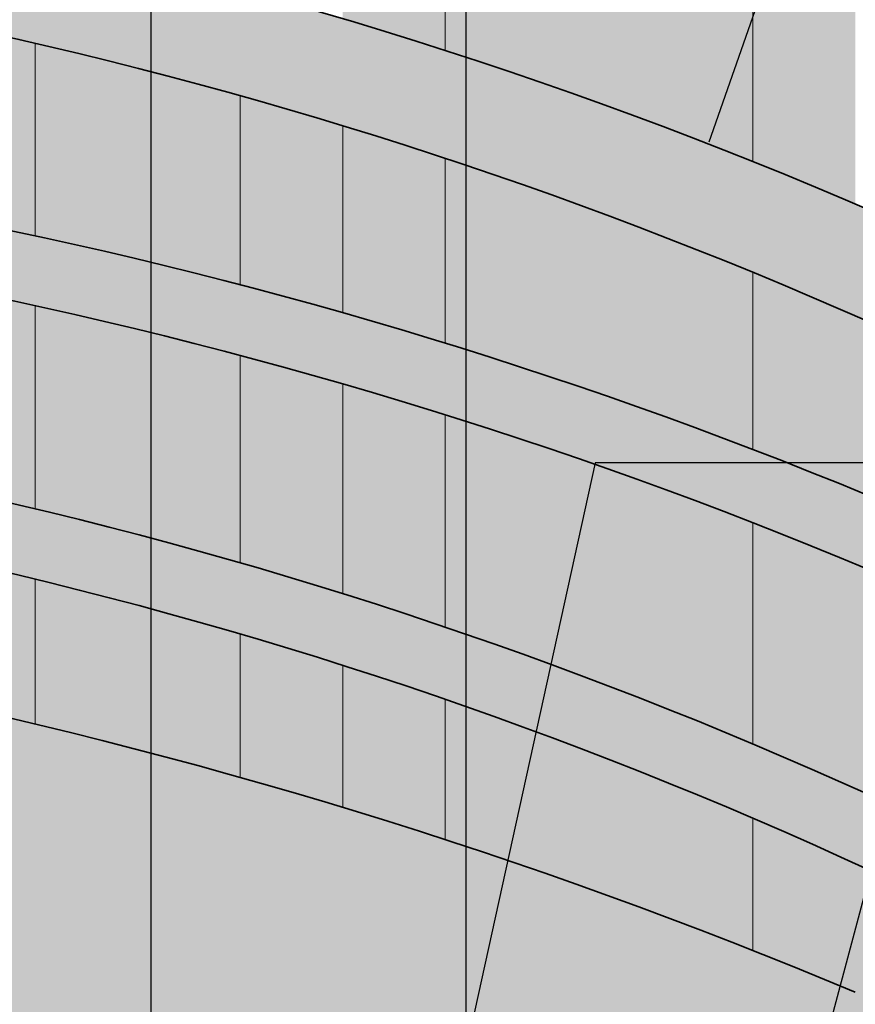
# Model space of a CAD drawing. Units: millimetres. Extents: x 130 to 1021, y 147 to 699.
# Tile 26 of 40: x 463 to 487, y 477 to 505. Entities that reach past the tile are written whole.
import ezdxf

# ---------------------------------------------------------------- set-up
doc = ezdxf.new("R2010")
doc.units = ezdxf.units.MM
doc.header["$MEASUREMENT"] = 0
for name, color, linetype, lineweight in [('A-ANNO-DIMS', 2, 'Continuous', 18), ('A-ELEV', 7, 'Continuous', 35), ('A-ELEV-PATT', 9, 'Continuous', 13), ('A-ELEV-RAIL', 6, 'Continuous', 18)]:
    doc.layers.add(name, color=color, linetype=linetype, lineweight=lineweight)
doc.styles.get("Standard").update_dxf_attribs({"font": 'arial.ttf'})
doc.dimstyles.get("Standard").update_dxf_attribs({"dimtxt": 20, "dimasz": 10, "dimexe": 10, "dimexo": 10, "dimgap": 5, "dimtad": 0, "dimtih": 1, "dimtoh": 1, "dimdec": 0, "dimzin": 0, "dimdsep": 46, "dimtxsty": 'Standard', "dimcen": 5, "dimadec": 0, "dimazin": 0, "dimtfac": 1, "dimtdec": 0, "dimtofl": 0, "dimtmove": 0, "dimatfit": 3, "dimfxl": 1, "dimtolj": 1, "dimtzin": 0, "dimarcsym": 0})

# ---------------------------------------------------------------- blocks, each defined once
blk = doc.blocks.new('*D11')
at = {"layer": 'A-ANNO-DIMS', "color": 0, "lineweight": -2, "transparency": 16777216}
for p, q in [((737.374, 648.699), (737.374, 149.739)), ((299.374, 566.947), (299.374, 149.739)), ((309.374, 159.739), (490.857, 159.739)), ((727.374, 159.739), (545.891, 159.739))]:
    blk.add_line(p, q, dxfattribs=at)
at = {"layer": 'A-ANNO-DIMS', "color": 0, "transparency": 16777216}
for points in [[(309.374, 161.406), (309.374, 158.073), (299.374, 159.739)], [(727.374, 161.406), (727.374, 158.073), (737.374, 159.739)]]:
    blk.add_solid(points, dxfattribs=at)
at = {"layer": 'Defpoints', "color": 0, "transparency": 16777216}
for p in [(737.374, 658.699), (299.374, 576.947), (737.374, 159.739)]:
    blk.add_point(p, dxfattribs=at)
at = {"layer": 'A-ANNO-DIMS', "color": 0, "transparency": 16777216, "insert": (518.374, 159.739), "char_height": 20, "attachment_point": 5}
blk.add_mtext('\\A1;438', dxfattribs=at)
blk = doc.blocks.new('*D12')
at = {"layer": 'A-ANNO-DIMS', "color": 0, "lineweight": -2, "transparency": 16777216}
for p, q in [((477.374, 661.947), (265.074, 661.947)), ((275.074, 651.947), (275.074, 438.205)), ((275.074, 194.039), (275.074, 407.782)), ((357.163, 184.039), (265.074, 184.039))]:
    blk.add_line(p, q, dxfattribs=at)
at = {"layer": 'A-ANNO-DIMS', "color": 0, "transparency": 16777216}
for points in [[(273.407, 651.947), (276.74, 651.947), (275.074, 661.947)], [(273.407, 194.039), (276.74, 194.039), (275.074, 184.039)]]:
    blk.add_solid(points, dxfattribs=at)
at = {"layer": 'Defpoints', "color": 0, "transparency": 16777216}
for p in [(275.074, 661.947), (487.374, 661.947), (367.163, 184.039)]:
    blk.add_point(p, dxfattribs=at)
at = {"layer": 'A-ANNO-DIMS', "color": 0, "transparency": 16777216, "insert": (275.074, 422.993), "char_height": 20, "attachment_point": 5}
blk.add_mtext('\\A1;477.9', dxfattribs=at)
blk = doc.blocks.new('*D17')
at = {"layer": 'A-ANNO-DIMS', "color": 0, "lineweight": -2, "transparency": 16777216}
for p, q in [((363.922, 579.884), (363.922, 696.247)), ((375.85, 490.216), (375.85, 696.247)), ((353.922, 686.247), (343.922, 686.247)), ((385.85, 686.247), (395.85, 686.247))]:
    blk.add_line(p, q, dxfattribs=at)
at = {"layer": 'A-ANNO-DIMS', "color": 0, "transparency": 16777216}
for points in [[(353.922, 687.914), (353.922, 684.581), (363.922, 686.247)], [(385.85, 687.914), (385.85, 684.581), (375.85, 686.247)]]:
    blk.add_solid(points, dxfattribs=at)
at = {"layer": 'Defpoints', "color": 0, "transparency": 16777216}
for p in [(375.85, 686.247), (363.922, 569.884), (375.85, 480.216)]:
    blk.add_point(p, dxfattribs=at)
at = {"layer": 'A-ANNO-DIMS', "color": 0, "transparency": 16777216, "insert": (441.444, 686.247), "char_height": 20, "attachment_point": 5}
blk.add_mtext('\\A1;11.928', dxfattribs=at)
blk = doc.blocks.new('*D18')
at = {"layer": 'A-ANNO-DIMS', "color": 0, "lineweight": -2, "transparency": 16777216}
for p, q in [((375.85, 490.216), (375.85, 696.247)), ((382.374, 388.947), (382.374, 696.247)), ((365.85, 686.247), (355.85, 686.247)), ((392.374, 686.247), (402.374, 686.247))]:
    blk.add_line(p, q, dxfattribs=at)
at = {"layer": 'A-ANNO-DIMS', "color": 0, "transparency": 16777216}
for points in [[(365.85, 687.914), (365.85, 684.581), (375.85, 686.247)], [(392.374, 687.914), (392.374, 684.581), (382.374, 686.247)]]:
    blk.add_solid(points, dxfattribs=at)
at = {"layer": 'Defpoints', "color": 0, "transparency": 16777216}
for p in [(382.374, 686.247), (375.85, 480.216), (382.374, 378.947)]:
    blk.add_point(p, dxfattribs=at)
at = {"layer": 'A-ANNO-DIMS', "color": 0, "transparency": 16777216, "insert": (441.132, 686.247), "char_height": 20, "attachment_point": 5}
blk.add_mtext('\\A1;6.524', dxfattribs=at)
blk = doc.blocks.new('*D19')
at = {"layer": 'A-ANNO-DIMS', "color": 0, "lineweight": -2, "transparency": 16777216}
for p, q in [((382.374, 388.947), (382.374, 696.247)), ((414.652, 510.881), (414.652, 696.247)), ((392.374, 686.247), (404.652, 686.247)), ((414.652, 686.247), (424.652, 686.247))]:
    blk.add_line(p, q, dxfattribs=at)
at = {"layer": 'A-ANNO-DIMS', "color": 0, "transparency": 16777216}
for points in [[(392.374, 687.914), (392.374, 684.581), (382.374, 686.247)], [(404.652, 687.914), (404.652, 684.581), (414.652, 686.247)]]:
    blk.add_solid(points, dxfattribs=at)
at = {"layer": 'Defpoints', "color": 0, "transparency": 16777216}
for p in [(414.652, 686.247), (414.652, 500.881), (382.374, 378.947)]:
    blk.add_point(p, dxfattribs=at)
at = {"layer": 'A-ANNO-DIMS', "color": 0, "transparency": 16777216, "insert": (463.411, 686.247), "char_height": 20, "attachment_point": 5}
blk.add_mtext('\\A1;32.28', dxfattribs=at)
blk = doc.blocks.new('*D20')
at = {"layer": 'A-ANNO-DIMS', "color": 0, "lineweight": -2, "transparency": 16777216}
for p, q in [((414.652, 510.881), (414.652, 696.247)), ((432.374, 388.947), (432.374, 696.247)), ((404.652, 686.247), (394.652, 686.247)), ((442.374, 686.247), (452.374, 686.247))]:
    blk.add_line(p, q, dxfattribs=at)
at = {"layer": 'A-ANNO-DIMS', "color": 0, "transparency": 16777216}
for points in [[(404.652, 687.914), (404.652, 684.581), (414.652, 686.247)], [(442.374, 687.914), (442.374, 684.581), (432.374, 686.247)]]:
    blk.add_solid(points, dxfattribs=at)
at = {"layer": 'Defpoints', "color": 0, "transparency": 16777216}
for p in [(432.374, 686.247), (414.652, 500.881), (432.374, 378.947)]:
    blk.add_point(p, dxfattribs=at)
at = {"layer": 'A-ANNO-DIMS', "color": 0, "transparency": 16777216, "insert": (490.075, 686.247), "char_height": 20, "attachment_point": 5}
blk.add_mtext('\\A1;17.72', dxfattribs=at)
blk = doc.blocks.new('*D21')
at = {"layer": 'A-ANNO-DIMS', "color": 0, "lineweight": -2, "transparency": 16777216}
for p, q in [((432.374, 388.947), (432.374, 696.247)), ((447.374, 656.947), (447.374, 696.247)), ((422.374, 686.247), (412.374, 686.247)), ((457.374, 686.247), (467.374, 686.247))]:
    blk.add_line(p, q, dxfattribs=at)
at = {"layer": 'A-ANNO-DIMS', "color": 0, "transparency": 16777216}
for points in [[(422.374, 687.914), (422.374, 684.581), (432.374, 686.247)], [(457.374, 687.914), (457.374, 684.581), (447.374, 686.247)]]:
    blk.add_solid(points, dxfattribs=at)
at = {"layer": 'Defpoints', "color": 0, "transparency": 16777216}
for p in [(447.374, 686.247), (447.374, 646.947), (432.374, 378.947)]:
    blk.add_point(p, dxfattribs=at)
at = {"layer": 'A-ANNO-DIMS', "color": 0, "transparency": 16777216, "insert": (485.832, 686.247), "char_height": 20, "attachment_point": 5}
blk.add_mtext('\\A1;15', dxfattribs=at)
blk = doc.blocks.new('*D22')
at = {"layer": 'A-ANNO-DIMS', "color": 0, "lineweight": -2, "transparency": 16777216}
for p, q in [((447.374, 656.947), (447.374, 696.247)), ((466.767, 403.947), (466.767, 696.247)), ((437.374, 686.247), (427.374, 686.247)), ((476.767, 686.247), (486.767, 686.247))]:
    blk.add_line(p, q, dxfattribs=at)
at = {"layer": 'A-ANNO-DIMS', "color": 0, "transparency": 16777216}
for points in [[(437.374, 687.914), (437.374, 684.581), (447.374, 686.247)], [(476.767, 687.914), (476.767, 684.581), (466.767, 686.247)]]:
    blk.add_solid(points, dxfattribs=at)
at = {"layer": 'Defpoints', "color": 0, "transparency": 16777216}
for p in [(466.767, 686.247), (447.374, 646.947), (466.767, 393.947)]:
    blk.add_point(p, dxfattribs=at)
at = {"layer": 'A-ANNO-DIMS', "color": 0, "transparency": 16777216, "insert": (532.34, 686.247), "char_height": 20, "attachment_point": 5}
blk.add_mtext('\\A1;19.393', dxfattribs=at)
blk = doc.blocks.new('*D23')
at = {"layer": 'A-ANNO-DIMS', "color": 0, "lineweight": -2, "transparency": 16777216}
for p, q in [((466.767, 403.947), (466.767, 696.247)), ((475.988, 209.039), (475.988, 696.247)), ((456.767, 686.247), (446.767, 686.247)), ((485.988, 686.247), (495.988, 686.247))]:
    blk.add_line(p, q, dxfattribs=at)
at = {"layer": 'A-ANNO-DIMS', "color": 0, "transparency": 16777216}
for points in [[(456.767, 687.914), (456.767, 684.581), (466.767, 686.247)], [(485.988, 687.914), (485.988, 684.581), (475.988, 686.247)]]:
    blk.add_solid(points, dxfattribs=at)
at = {"layer": 'Defpoints', "color": 0, "transparency": 16777216}
for p in [(475.988, 686.247), (466.767, 393.947), (475.988, 199.039)]:
    blk.add_point(p, dxfattribs=at)
at = {"layer": 'A-ANNO-DIMS', "color": 0, "transparency": 16777216, "insert": (534.631, 686.247), "char_height": 20, "attachment_point": 5}
blk.add_mtext('\\A1;9.222', dxfattribs=at)
blk = doc.blocks.new('*D24')
at = {"layer": 'A-ANNO-DIMS', "color": 0, "lineweight": -2, "transparency": 16777216}
for p, q in [((475.988, 209.039), (475.988, 696.247)), ((487.374, 671.947), (487.374, 696.247)), ((465.988, 686.247), (455.988, 686.247)), ((497.374, 686.247), (507.374, 686.247))]:
    blk.add_line(p, q, dxfattribs=at)
at = {"layer": 'A-ANNO-DIMS', "color": 0, "transparency": 16777216}
for points in [[(465.988, 687.914), (465.988, 684.581), (475.988, 686.247)], [(497.374, 687.914), (497.374, 684.581), (487.374, 686.247)]]:
    blk.add_solid(points, dxfattribs=at)
at = {"layer": 'Defpoints', "color": 0, "transparency": 16777216}
for p in [(487.374, 686.247), (487.374, 661.947), (475.988, 199.039)]:
    blk.add_point(p, dxfattribs=at)
at = {"layer": 'A-ANNO-DIMS', "color": 0, "transparency": 16777216, "insert": (553.022, 686.247), "char_height": 20, "attachment_point": 5}
blk.add_mtext('\\A1;11.385', dxfattribs=at)
blk = doc.blocks.new('*D25')
at = {"layer": 'A-ANNO-DIMS', "color": 0, "lineweight": -2, "transparency": 16777216}
for p, q in [((487.374, 671.947), (487.374, 696.247)), ((494.102, 506.908), (494.102, 696.247)), ((477.374, 686.247), (467.374, 686.247)), ((504.102, 686.247), (514.102, 686.247))]:
    blk.add_line(p, q, dxfattribs=at)
at = {"layer": 'A-ANNO-DIMS', "color": 0, "transparency": 16777216}
for points in [[(477.374, 687.914), (477.374, 684.581), (487.374, 686.247)], [(504.102, 687.914), (504.102, 684.581), (494.102, 686.247)]]:
    blk.add_solid(points, dxfattribs=at)
at = {"layer": 'Defpoints', "color": 0, "transparency": 16777216}
for p in [(494.102, 686.247), (487.374, 661.947), (494.102, 496.908)]:
    blk.add_point(p, dxfattribs=at)
at = {"layer": 'A-ANNO-DIMS', "color": 0, "transparency": 16777216, "insert": (552.922, 686.247), "char_height": 20, "attachment_point": 5}
blk.add_mtext('\\A1;6.728', dxfattribs=at)
blk = doc.blocks.new('*D26')
at = {"layer": 'A-ANNO-DIMS', "color": 0, "lineweight": -2, "transparency": 16777216}
for p, q in [((494.102, 506.908), (494.102, 696.247)), ((502.374, 593.947), (502.374, 696.247)), ((484.102, 686.247), (474.102, 686.247)), ((512.374, 686.247), (522.374, 686.247))]:
    blk.add_line(p, q, dxfattribs=at)
at = {"layer": 'A-ANNO-DIMS', "color": 0, "transparency": 16777216}
for points in [[(484.102, 687.914), (484.102, 684.581), (494.102, 686.247)], [(512.374, 687.914), (512.374, 684.581), (502.374, 686.247)]]:
    blk.add_solid(points, dxfattribs=at)
at = {"layer": 'Defpoints', "color": 0, "transparency": 16777216}
for p in [(502.374, 686.247), (502.374, 583.947), (494.102, 496.908)]:
    blk.add_point(p, dxfattribs=at)
at = {"layer": 'A-ANNO-DIMS', "color": 0, "transparency": 16777216, "insert": (561.03, 686.247), "char_height": 20, "attachment_point": 5}
blk.add_mtext('\\A1;8.272', dxfattribs=at)
blk = doc.blocks.new('*D65')
at = {"layer": 'A-ANNO-DIMS', "color": 0, "lineweight": -2, "transparency": 16777216}
for p, q in [((495.463, 509.127), (472.508, 423.108)), ((505.463, 509.127), (495.463, 509.127)), ((427.374, 248.979), (427.374, 258.979)), ((422.374, 253.979), (432.374, 253.979))]:
    blk.add_line(p, q, dxfattribs=at)
at = {"layer": 'A-ANNO-DIMS', "color": 0, "transparency": 16777216}
blk.add_solid([(470.898, 423.538), (474.118, 422.679), (469.93, 413.447)], dxfattribs=at)
at = {"layer": 'Defpoints', "color": 0, "transparency": 16777216}
for p in [(469.93, 413.447), (427.374, 253.979)]:
    blk.add_point(p, dxfattribs=at)
at = {"layer": 'A-ANNO-DIMS', "color": 0, "transparency": 16777216, "insert": (561.623, 509.127), "char_height": 20, "attachment_point": 5}
blk.add_mtext('\\A1;R165.05', dxfattribs=at)
blk = doc.blocks.new('*D67')
at = {"layer": 'A-ANNO-DIMS', "color": 0, "lineweight": -2, "transparency": 16777216}
for p, q in [((479.756, 492.431), (462.144, 412.223)), ((489.756, 492.431), (479.756, 492.431)), ((427.07, 247.496), (427.07, 257.496)), ((422.07, 252.496), (432.07, 252.496))]:
    blk.add_line(p, q, dxfattribs=at)
at = {"layer": 'A-ANNO-DIMS', "color": 0, "transparency": 16777216}
blk.add_solid([(460.516, 412.58), (463.772, 411.865), (459.999, 402.455)], dxfattribs=at)
at = {"layer": 'Defpoints', "color": 0, "transparency": 16777216}
for p in [(459.999, 402.455), (427.07, 252.496)]:
    blk.add_point(p, dxfattribs=at)
at = {"layer": 'A-ANNO-DIMS', "color": 0, "transparency": 16777216, "insert": (545.841, 492.431), "char_height": 20, "attachment_point": 5}
blk.add_mtext('\\A1;R153.53', dxfattribs=at)
blk = doc.blocks.new('*D69')
at = {"layer": 'A-ANNO-DIMS', "color": 0, "lineweight": -2, "transparency": 16777216}
for p, q in [((507.746, 572.261), (483.091, 501.813)), ((517.746, 572.261), (507.746, 572.261)), ((433.191, 354.23), (433.191, 364.23)), ((428.191, 359.23), (438.191, 359.23))]:
    blk.add_line(p, q, dxfattribs=at)
at = {"layer": 'A-ANNO-DIMS', "color": 0, "transparency": 16777216}
blk.add_solid([(481.518, 502.363), (484.664, 501.262), (479.788, 492.374)], dxfattribs=at)
at = {"layer": 'Defpoints', "color": 0, "transparency": 16777216}
for p in [(479.788, 492.374), (433.191, 359.23)]:
    blk.add_point(p, dxfattribs=at)
at = {"layer": 'A-ANNO-DIMS', "color": 0, "transparency": 16777216, "insert": (573.824, 572.261), "char_height": 20, "attachment_point": 5}
blk.add_mtext('\\A1;R141.06', dxfattribs=at)
blk = doc.blocks.new('*D71')
at = {"layer": 'A-ANNO-DIMS', "color": 0, "lineweight": -2, "transparency": 16777216}
for p, q in [((492.108, 581.609), (472.542, 512.666)), ((502.108, 581.609), (492.108, 581.609)), ((432.65, 367.109), (432.65, 377.109)), ((427.65, 372.109), (437.65, 372.109))]:
    blk.add_line(p, q, dxfattribs=at)
at = {"layer": 'A-ANNO-DIMS', "color": 0, "transparency": 16777216}
blk.add_solid([(470.938, 513.121), (474.145, 512.211), (469.812, 503.046)], dxfattribs=at)
at = {"layer": 'Defpoints', "color": 0, "transparency": 16777216}
for p in [(469.812, 503.046), (432.65, 372.109)]:
    blk.add_point(p, dxfattribs=at)
at = {"layer": 'A-ANNO-DIMS', "color": 0, "transparency": 16777216, "insert": (548.493, 581.609), "char_height": 20, "attachment_point": 5}
blk.add_mtext('\\A1;R136.1', dxfattribs=at)
blk = doc.blocks.new('*D72')
at = {"layer": 'A-ANNO-DIMS', "color": 0, "lineweight": -2, "transparency": 16777216}
for p, q in [((460.658, 573.64), (451.279, 503.49)), ((470.658, 573.64), (460.658, 573.64)), ((432.115, 355.142), (432.115, 365.142)), ((427.115, 360.142), (437.115, 360.142))]:
    blk.add_line(p, q, dxfattribs=at)
at = {"layer": 'A-ANNO-DIMS', "color": 0, "transparency": 16777216}
blk.add_solid([(449.628, 503.711), (452.931, 503.27), (449.954, 493.579)], dxfattribs=at)
at = {"layer": 'Defpoints', "color": 0, "transparency": 16777216}
for p in [(449.954, 493.579), (432.115, 360.142)]:
    blk.add_point(p, dxfattribs=at)
at = {"layer": 'A-ANNO-DIMS', "color": 0, "transparency": 16777216, "insert": (526.64, 573.64), "char_height": 20, "attachment_point": 5}
blk.add_mtext('\\A1;R134.62', dxfattribs=at)

msp = doc.modelspace()

# ---------------------------------------------------------------- hatches: boundary and pattern name
at = {"layer": 'A-ELEV-PATT'}
h = msp.add_hatch(color=256, dxfattribs=at)
h.dxf.hatch_style = 1
h.paths.add_polyline_path([(737.3738, 658.6988, 0.0135961), (632.4019, 661.9473), (607.3738, 661.9473), (487.3738, 661.9473), (487.3738, 649.9473), (607.3738, 649.9473), (632.3794, 649.9473, -0.0136841), (737.3738, 646.6784)])
h.paths.add_polyline_path([(732.3738, 643.9599, 0.0130529), (632.3738, 646.9473), (607.3738, 646.9473), (487.3738, 646.9473), (487.3738, 596.9473), (632.3738, 596.9473, -0.0130529), (732.3738, 593.9599)])
h.paths.add_polyline_path([(737.3738, 593.6732, 0.0137063), (632.3738, 596.9473), (487.3738, 596.9473), (487.3738, 586.9473), (632.355, 586.9473, -0.0137808), (737.3738, 583.6559)])
h.paths.add_polyline_path([(447.3738, 646.9473), (307.3738, 646.9473), (302.3738, 646.9473), (302.3738, 634.9473), (447.3738, 634.9473)])
h.paths.add_polyline_path([(447.3738, 631.9473), (307.3738, 631.9473), (307.3738, 586.9473), (447.3738, 586.9473)])
h.paths.add_polyline_path([(447.3738, 586.9473), (307.3738, 586.9473), (302.3738, 586.9473), (302.3738, 576.9473), (447.3738, 576.9473)])
h.paths.add_polyline_path([(447.3738, 573.9473), (367.3738, 573.9473), (367.3738, 539.9473), (447.3738, 539.9473)])
h.paths.add_polyline_path([(447.3738, 537.9473), (367.3738, 537.9473), (367.3738, 507.9473), (400.392, 507.4253, -0.001728), (401.3281, 507.6451, -0.5220025), (425.6117, 511.0391, -0.0391849), (447.3738, 510.4359), (447.3738, 510.7883)])
h.paths.add_polyline_path([(394.7238, 505.9473), (367.3738, 505.9473), (367.3738, 476.9473, -0.0146512), (375.8501, 480.2159), (376.1506, 499.2266, -0.0355419)])
h.paths.add_polyline_path([(632.3738, 583.9473), (552.3738, 583.9473), (552.3738, 550.9473), (632.3738, 550.9473)])
h.paths.add_polyline_path([(632.3738, 548.9473), (552.3738, 548.9473), (552.3738, 515.9473), (632.3738, 515.9473)])
h.paths.add_polyline_path([(632.3738, 513.9473), (552.3738, 513.9473), (552.3738, 476.9473), (632.3738, 476.9473)])
h.paths.add_polyline_path([(737.3738, 473.6903, 0.0136326), (632.3926, 476.9473), (552.3738, 476.9473), (487.3738, 476.9473), (487.3738, 466.9473), (632.3738, 466.9473, -0.0137063), (737.3738, 463.6732)])
h.paths.add_polyline_path([(732.3738, 460.9552, 0.0130741), (632.3681, 463.9473), (487.3738, 463.9473), (487.3738, 407.735, -0.0032286), (489.3544, 406.9473), (632.3926, 406.9473, -0.0129826), (732.3738, 403.9755)])
h.paths.add_polyline_path([(487.3738, 463.9473, 0.20133), (367.3738, 463.9473), (367.3738, 407.735, -0.1882031), (487.3738, 407.735)])
h.paths.add_polyline_path([(367.3738, 476.9473), (367.3738, 466.9473, -0.2013309), (487.3738, 466.9473), (487.3738, 476.9473, 0.20133)])
h.paths.add_polyline_path([(367.3738, 463.9473), (307.3738, 463.9473), (307.3738, 401.9473), (357.9413, 401.9473), (367.3738, 407.735)])
h.paths.add_polyline_path([(367.3738, 476.9473), (302.3738, 476.9473), (302.3738, 466.9473), (367.3738, 466.9473)])
h.paths.add_polyline_path([(632.8184, 366.9453), (552.3738, 366.9453), (552.3738, 393.9473), (632.8184, 393.9473)])
h.paths.add_polyline_path([(632.8184, 357.2114), (632.8184, 363.9453), (552.3738, 363.9453), (552.3738, 357.2114), (552.3738, 336.9453), (632.8184, 336.9453)])
h.paths.add_polyline_path([(632.8184, 333.9453), (552.3738, 333.9453), (552.3738, 306.9453), (632.8184, 306.9453)])
h.paths.add_polyline_path([(632.8184, 303.9453), (552.3738, 303.9453), (552.3738, 273.9473), (632.355, 273.9473, 0.0000608), (632.8184, 273.9491)])
h.paths.add_polyline_path([(737.3738, 403.6903, 0.0136326), (632.3926, 406.9473), (489.3544, 406.9473, 0.1915481), (367.3738, 407.735), (367.3738, 396.9473, -0.2013309), (487.3738, 396.9473), (632.3738, 396.9473, -0.0137063), (737.3738, 393.6732)])
h.paths.add_polyline_path([(357.9413, 401.9473), (307.3738, 401.9473), (307.3738, 391.9473), (357.9413, 391.9473)])
h.paths.add_polyline_path([(357.9413, 357.2114), (357.9413, 388.9473), (307.3738, 388.9473), (307.3738, 357.2114), (307.3738, 273.9473), (357.9413, 273.9473)])
h.paths.add_polyline_path([(732.3738, 263.93, -0.0130317), (632.3794, 260.9473), (466.7667, 260.9473), (466.7667, 240.9473), (469.8406, 236.978), (469.8406, 221.978), (472.9145, 218.0087), (472.9145, 213.9473), (607.3738, 213.9473), (732.3738, 213.9473)])
h.paths.add_polyline_path([(732.3738, 290.889), (722.479, 290.889), (722.479, 301.889), (732.3738, 301.889), (732.3738, 305.889), (722.479, 305.889), (722.479, 316.889), (732.3738, 316.889), (732.3738, 320.889), (722.479, 320.889), (722.479, 331.889), (732.3738, 331.889), (732.3738, 335.889), (722.479, 335.889), (722.479, 346.889), (732.3738, 346.889), (732.3738, 350.889), (722.479, 350.889), (722.479, 361.889), (732.3738, 361.889), (732.3738, 365.889), (722.479, 365.889), (722.479, 376.889), (732.3738, 376.889), (732.3738, 380.889), (722.479, 380.889), (722.479, 391.4848, 0.0005233), (718.479, 391.6843), (718.479, 380.889), (707.479, 380.889), (707.479, 392.1896, 0.0005231), (703.479, 392.3576), (703.479, 380.889), (692.479, 380.889), (692.479, 392.7765, 0.0005229), (688.479, 392.9131), (688.479, 380.889), (677.479, 380.889), (677.479, 393.2456, 0.0005228), (673.479, 393.3508), (673.479, 380.889), (662.479, 380.889), (662.479, 393.597, 0.0005227), (658.479, 393.6709), (658.479, 380.889), (647.479, 380.889), (647.479, 393.8308, 0.0005226), (643.479, 393.8732), (643.479, 380.889), (632.8184, 380.889), (632.8184, 376.889), (643.479, 376.889), (643.479, 365.889), (632.8184, 365.889), (632.8184, 361.889), (643.479, 361.889), (643.479, 350.889), (632.8184, 350.889), (632.8184, 346.889), (643.479, 346.889), (643.479, 335.889), (632.8184, 335.889), (632.8184, 331.889), (643.479, 331.889), (643.479, 320.889), (632.8184, 320.889), (632.8184, 316.889), (643.479, 316.889), (643.479, 305.889), (632.8184, 305.889), (632.8184, 301.889), (643.479, 301.889), (643.479, 290.889), (632.8184, 290.889), (632.8184, 286.889), (643.479, 286.889), (643.479, 274.0217, 0.0005246), (647.479, 274.0643), (647.479, 286.889), (658.479, 286.889), (658.479, 274.2248, 0.0005246), (662.479, 274.2989), (662.479, 286.889), (673.479, 286.889), (673.479, 274.546, 0.0005247), (677.479, 274.6516), (677.479, 286.889), (688.479, 286.889), (688.479, 274.9853, 0.0005248), (692.479, 275.1224), (692.479, 286.889), (703.479, 286.889), (703.479, 275.5429, 0.000525), (707.479, 275.7115), (707.479, 286.889), (718.479, 286.889), (718.479, 276.2187, 0.0005252), (722.479, 276.4189), (722.479, 286.889), (732.3738, 286.889)])
h.paths.add_polyline_path([(718.479, 290.889), (707.479, 290.889), (707.479, 301.889), (718.479, 301.889)], flags=16)
h.paths.add_polyline_path([(703.479, 290.889), (692.479, 290.889), (692.479, 301.889), (703.479, 301.889)], flags=16)
h.paths.add_polyline_path([(718.479, 305.889), (707.479, 305.889), (707.479, 316.889), (718.479, 316.889)], flags=16)
h.paths.add_polyline_path([(703.479, 305.889), (692.479, 305.889), (692.479, 316.889), (703.479, 316.889)], flags=16)
h.paths.add_polyline_path([(688.479, 290.889), (677.479, 290.889), (677.479, 301.889), (688.479, 301.889)], flags=16)
h.paths.add_polyline_path([(718.479, 320.889), (707.479, 320.889), (707.479, 331.889), (718.479, 331.889)], flags=16)
h.paths.add_polyline_path([(688.479, 305.889), (677.479, 305.889), (677.479, 316.889), (688.479, 316.889)], flags=16)
h.paths.add_polyline_path([(703.479, 320.889), (692.479, 320.889), (692.479, 331.889), (703.479, 331.889)], flags=16)
h.paths.add_polyline_path([(688.479, 320.889), (677.479, 320.889), (677.479, 331.889), (688.479, 331.889)], flags=16)
h.paths.add_polyline_path([(673.479, 290.889), (662.479, 290.889), (662.479, 301.889), (673.479, 301.889)], flags=16)
h.paths.add_polyline_path([(718.479, 335.889), (707.479, 335.889), (707.479, 346.889), (718.479, 346.889)], flags=16)
h.paths.add_polyline_path([(673.479, 305.889), (662.479, 305.889), (662.479, 316.889), (673.479, 316.889)], flags=16)
h.paths.add_polyline_path([(703.479, 335.889), (692.479, 335.889), (692.479, 346.889), (703.479, 346.889)], flags=16)
h.paths.add_polyline_path([(673.479, 320.889), (662.479, 320.889), (662.479, 331.889), (673.479, 331.889)], flags=16)
h.paths.add_polyline_path([(688.479, 335.889), (677.479, 335.889), (677.479, 346.889), (688.479, 346.889)], flags=16)
h.paths.add_polyline_path([(658.479, 290.889), (647.479, 290.889), (647.479, 301.889), (658.479, 301.889)], flags=16)
h.paths.add_polyline_path([(718.479, 350.889), (707.479, 350.889), (707.479, 361.889), (718.479, 361.889)], flags=16)
h.paths.add_polyline_path([(658.479, 305.889), (647.479, 305.889), (647.479, 316.889), (658.479, 316.889)], flags=16)
h.paths.add_polyline_path([(703.479, 350.889), (692.479, 350.889), (692.479, 361.889), (703.479, 361.889)], flags=16)
h.paths.add_polyline_path([(673.479, 335.889), (662.479, 335.889), (662.479, 346.889), (673.479, 346.889)], flags=16)
h.paths.add_polyline_path([(658.479, 320.889), (647.479, 320.889), (647.479, 331.889), (658.479, 331.889)], flags=16)
h.paths.add_polyline_path([(688.479, 350.889), (677.479, 350.889), (677.479, 361.889), (688.479, 361.889)], flags=16)
h.paths.add_polyline_path([(718.479, 365.889), (707.479, 365.889), (707.479, 376.889), (718.479, 376.889)], flags=16)
h.paths.add_polyline_path([(658.479, 335.889), (647.479, 335.889), (647.479, 346.889), (658.479, 346.889)], flags=16)
h.paths.add_polyline_path([(673.479, 350.889), (662.479, 350.889), (662.479, 361.889), (673.479, 361.889)], flags=16)
h.paths.add_polyline_path([(703.479, 365.889), (692.479, 365.889), (692.479, 376.889), (703.479, 376.889)], flags=16)
h.paths.add_polyline_path([(688.479, 365.889), (677.479, 365.889), (677.479, 376.889), (688.479, 376.889)], flags=16)
h.paths.add_polyline_path([(658.479, 350.889), (647.479, 350.889), (647.479, 361.889), (658.479, 361.889)], flags=16)
h.paths.add_polyline_path([(673.479, 365.889), (662.479, 365.889), (662.479, 376.889), (673.479, 376.889)], flags=16)
h.paths.add_polyline_path([(658.479, 365.889), (647.479, 365.889), (647.479, 376.889), (658.479, 376.889)], flags=16)
h.paths.add_polyline_path([(732.3738, 503.9786), (722.3392, 503.9786), (722.3392, 514.9786), (732.3738, 514.9786), (732.3738, 518.9786), (722.3392, 518.9786), (722.3392, 529.9786), (732.3738, 529.9786), (732.3738, 533.9786), (722.3392, 533.9786), (722.3392, 544.9786), (732.3738, 544.9786), (732.3738, 546.9473), (732.3738, 548.9786), (722.3392, 548.9786), (722.3392, 559.9786), (732.3738, 559.9786), (732.3738, 563.9786), (722.3392, 563.9786), (722.3392, 574.9786), (732.3738, 574.9786), (732.3738, 578.9786), (722.3392, 578.9786), (722.3392, 581.4789, 0.000526), (718.3392, 581.6791), (718.3392, 578.9786), (707.3392, 578.9786), (707.3392, 582.1863, 0.0005258), (703.3392, 582.355), (703.3392, 578.9786), (692.3392, 578.9786), (692.3392, 582.7752, 0.0005257), (688.3392, 582.9123), (688.3392, 578.9786), (677.3392, 578.9786), (677.3392, 583.2457, 0.0005255), (673.3392, 583.3512), (673.3392, 578.9786), (662.3392, 578.9786), (662.3392, 583.5978, 0.0005254), (658.3392, 583.6718), (658.3392, 578.9786), (647.3392, 578.9786), (647.3392, 583.8317, 0.0005254), (643.3392, 583.8741), (643.3392, 578.9786), (632.3738, 578.9786), (632.3738, 574.9786), (643.3392, 574.9786), (643.3392, 563.9786), (632.3738, 563.9786), (632.3738, 559.9786), (643.3392, 559.9786), (643.3392, 548.9786), (632.3738, 548.9786), (632.3738, 544.9786), (643.3392, 544.9786), (643.3392, 533.9786), (632.3738, 533.9786), (632.3738, 529.9786), (643.3392, 529.9786), (643.3392, 518.9786), (632.3738, 518.9786), (632.3738, 515.9473), (632.3738, 514.9786), (643.3392, 514.9786), (643.3392, 503.9786), (632.3738, 503.9786), (632.3738, 499.9786), (643.3392, 499.9786), (643.3392, 488.9786), (632.3738, 488.9786), (632.3738, 484.9786), (643.3392, 484.9786), (643.3392, 476.8751, -0.0005191), (647.3392, 476.8332), (647.3392, 484.9786), (658.3392, 484.9786), (658.3392, 476.6752, -0.0005192), (662.3392, 476.6022), (662.3392, 484.9786), (673.3392, 484.9786), (673.3392, 476.3585, -0.0005193), (677.3392, 476.2543), (677.3392, 484.9786), (688.3392, 484.9786), (688.3392, 475.9248, -0.0005194), (692.3392, 475.7894), (692.3392, 484.9786), (703.3392, 484.9786), (703.3392, 475.3741, -0.0005195), (707.3392, 475.2075), (707.3392, 484.9786), (718.3392, 484.9786), (718.3392, 474.7064, -0.0005197), (722.3392, 474.5086), (722.3392, 484.9786), (732.3738, 484.9786), (732.3738, 488.9786), (722.3392, 488.9786), (722.3392, 499.9786), (732.3738, 499.9786)])
h.paths.add_polyline_path([(718.3392, 503.9786), (707.3392, 503.9786), (707.3392, 514.9786), (718.3392, 514.9786)], flags=16)
h.paths.add_polyline_path([(718.3392, 499.9786), (718.3392, 488.9786), (707.3392, 488.9786), (707.3392, 499.9786)], flags=16)
h.paths.add_polyline_path([(718.3392, 518.9786), (707.3392, 518.9786), (707.3392, 529.9786), (718.3392, 529.9786)], flags=16)
h.paths.add_polyline_path([(703.3392, 503.9786), (692.3392, 503.9786), (692.3392, 514.9786), (703.3392, 514.9786)], flags=16)
h.paths.add_polyline_path([(703.3392, 499.9786), (703.3392, 488.9786), (692.3392, 488.9786), (692.3392, 499.9786)], flags=16)
h.paths.add_polyline_path([(703.3392, 518.9786), (692.3392, 518.9786), (692.3392, 529.9786), (703.3392, 529.9786)], flags=16)
h.paths.add_polyline_path([(718.3392, 533.9786), (707.3392, 533.9786), (707.3392, 544.9786), (718.3392, 544.9786)], flags=16)
h.paths.add_polyline_path([(688.3392, 503.9786), (677.3392, 503.9786), (677.3392, 514.9786), (688.3392, 514.9786)], flags=16)
h.paths.add_polyline_path([(688.3392, 499.9786), (688.3392, 488.9786), (677.3392, 488.9786), (677.3392, 499.9786)], flags=16)
h.paths.add_polyline_path([(703.3392, 533.9786), (692.3392, 533.9786), (692.3392, 544.9786), (703.3392, 544.9786)], flags=16)
h.paths.add_polyline_path([(688.3392, 518.9786), (677.3392, 518.9786), (677.3392, 529.9786), (688.3392, 529.9786)], flags=16)
h.paths.add_polyline_path([(688.3392, 533.9786), (677.3392, 533.9786), (677.3392, 544.9786), (688.3392, 544.9786)], flags=16)
h.paths.add_polyline_path([(718.3392, 548.9786), (707.3392, 548.9786), (707.3392, 559.9786), (718.3392, 559.9786)], flags=16)
h.paths.add_polyline_path([(673.3392, 503.9786), (662.3392, 503.9786), (662.3392, 514.9786), (673.3392, 514.9786)], flags=16)
h.paths.add_polyline_path([(673.3392, 499.9786), (673.3392, 488.9786), (662.3392, 488.9786), (662.3392, 499.9786)], flags=16)
h.paths.add_polyline_path([(703.3392, 548.9786), (692.3392, 548.9786), (692.3392, 559.9786), (703.3392, 559.9786)], flags=16)
h.paths.add_polyline_path([(673.3392, 518.9786), (662.3392, 518.9786), (662.3392, 529.9786), (673.3392, 529.9786)], flags=16)
h.paths.add_polyline_path([(688.3392, 548.9786), (677.3392, 548.9786), (677.3392, 559.9786), (688.3392, 559.9786)], flags=16)
h.paths.add_polyline_path([(673.3392, 533.9786), (662.3392, 533.9786), (662.3392, 544.9786), (673.3392, 544.9786)], flags=16)
h.paths.add_polyline_path([(718.3392, 563.9786), (707.3392, 563.9786), (707.3392, 574.9786), (718.3392, 574.9786)], flags=16)
h.paths.add_polyline_path([(658.3392, 503.9786), (647.3392, 503.9786), (647.3392, 514.9786), (658.3392, 514.9786)], flags=16)
h.paths.add_polyline_path([(658.3392, 499.9786), (658.3392, 488.9786), (647.3392, 488.9786), (647.3392, 499.9786)], flags=16)
h.paths.add_polyline_path([(703.3392, 563.9786), (692.3392, 563.9786), (692.3392, 574.9786), (703.3392, 574.9786)], flags=16)
h.paths.add_polyline_path([(658.3392, 518.9786), (647.3392, 518.9786), (647.3392, 529.9786), (658.3392, 529.9786)], flags=16)
h.paths.add_polyline_path([(673.3392, 548.9786), (662.3392, 548.9786), (662.3392, 559.9786), (673.3392, 559.9786)], flags=16)
h.paths.add_polyline_path([(688.3392, 563.9786), (677.3392, 563.9786), (677.3392, 574.9786), (688.3392, 574.9786)], flags=16)
h.paths.add_polyline_path([(658.3392, 533.9786), (647.3392, 533.9786), (647.3392, 544.9786), (658.3392, 544.9786)], flags=16)
h.paths.add_polyline_path([(673.3392, 563.9786), (662.3392, 563.9786), (662.3392, 574.9786), (673.3392, 574.9786)], flags=16)
h.paths.add_polyline_path([(658.3392, 548.9786), (647.3392, 548.9786), (647.3392, 559.9786), (658.3392, 559.9786)], flags=16)
h.paths.add_polyline_path([(658.3392, 563.9786), (647.3392, 563.9786), (647.3392, 574.9786), (658.3392, 574.9786)], flags=16)
h = msp.add_hatch(color=256, dxfattribs=at)
h.dxf.hatch_style = 1
h.paths.add_polyline_path([(447.3738, 576.9473), (302.3738, 576.9473), (302.3738, 573.9473), (447.3738, 573.9473)])
h.paths.add_polyline_path([(487.3738, 583.9473), (487.3738, 586.9473), (447.3738, 576.9473), (447.3738, 573.9473)])
h.paths.add_polyline_path([(632.355, 586.9473), (487.3738, 586.9473), (487.3738, 583.9473), (632.3738, 583.9473), (632.3738, 583.9472, -0.0138), (737.3738, 580.6507), (737.3738, 583.6559, 0.0137808)])
h.paths.add_polyline_path([(367.3738, 466.9473), (302.3738, 466.9473), (302.3738, 463.9473), (367.3738, 463.9473)])
h.paths.add_polyline_path([(487.3738, 463.9473), (487.3738, 466.9473, 0.2013309), (367.3738, 466.9473), (367.3738, 463.9473, -0.20133)])
h.paths.add_polyline_path([(632.3738, 466.9473), (487.3738, 466.9473), (487.3738, 463.9473), (632.3681, 463.9473, -0.0137285), (737.3738, 460.6681), (737.3738, 463.6732, 0.0137063)])
h.paths.add_polyline_path([(632.3738, 396.9473), (487.3738, 396.9473, 0.2013309), (367.3738, 396.9473), (367.3738, 393.9473, -0.2023717), (486.7667, 393.9473), (632.3681, 393.9473, -0.0137285), (737.3738, 390.6681), (737.3738, 393.6732, 0.0137063)])
h.paths.add_polyline_path([(357.9413, 391.9473), (307.3738, 391.9473), (307.3738, 388.9473), (357.9413, 388.9473)])
h.paths.add_polyline_path([(367.3738, 393.9473), (367.3738, 396.9473), (357.9413, 391.924), (357.9413, 388.9473), (358.058, 388.9473)])
h.paths.add_polyline_path([(737.3738, 264.2162), (737.3738, 267.2214, -0.0137063), (632.3738, 263.9473), (463.7667, 263.9473), (466.7667, 260.9473), (632.3794, 260.9473, 0.0136841)])
h.paths.add_polyline_path([(463.7667, 263.9473), (447.3738, 263.9473), (450.3738, 260.9473), (466.7667, 260.9473)])
h.paths.add_polyline_path([(447.3738, 263.9473), (432.3738, 263.9473), (432.3738, 260.9473), (450.3738, 260.9473)])
h.paths.add_polyline_path([(382.3738, 263.9473), (357.9413, 263.9473), (357.9413, 260.9473), (382.3738, 260.9473)])
h.paths.add_polyline_path([(357.9413, 263.9473), (307.3738, 263.9473), (307.3738, 260.9473), (357.9413, 260.9473)])
h = msp.add_hatch(color=256, dxfattribs=at)
h.paths.add_polyline_path([(327.3738, 569.884), (327.3738, 573.9473), (307.3738, 573.9473), (307.3738, 476.9473), (327.3738, 476.9473), (327.3738, 480.95)])
h.paths.add_polyline_path([(486.7667, 386.2639), (486.7667, 393.9473), (466.7667, 393.9473), (466.7667, 357.2114), (466.7667, 311.9335, 0.0342703), (486.7667, 308.4637)])
h.paths.add_polyline_path([(486.7667, 308.4637, -0.0342703), (466.7667, 311.9335), (466.7667, 273.9473), (486.7667, 273.9473)])
h.paths.add_polyline_path([(389.3738, 351.5473), (396.7693, 351.5473, -0.007027), (393.8774, 354.5473), (389.3738, 354.5473), (389.3738, 359.5775, -0.0190302), (382.3738, 368.424), (382.3738, 249.5473), (432.3738, 249.5473), (432.3738, 325.067, -0.0057673), (429.3738, 326.709), (429.3738, 257.5473), (426.3738, 257.5473), (426.3738, 328.4428, -0.0059254), (423.3738, 330.272), (423.3738, 315.7473), (389.3738, 315.7473), (389.3738, 332.1473), (420.4552, 332.1473, -0.008951), (416.0768, 335.1473), (389.3738, 335.1473)])
h.paths.add_polyline_path([(389.3738, 312.7473), (423.3738, 312.7473), (423.3738, 296.3473), (389.3738, 296.3473)], flags=16)
h.paths.add_polyline_path([(389.3738, 293.3473), (423.3738, 293.3473), (423.3738, 276.9473), (389.3738, 276.9473)], flags=16)
h.paths.add_polyline_path([(389.3738, 273.9473), (423.3738, 273.9473), (423.3738, 257.5473), (389.3738, 257.5473)], flags=16)
h.paths.add_polyline_path([(432.3738, 378.9473), (382.3738, 378.9473), (382.3738, 368.424, 0.0190302), (389.3738, 359.5775), (389.3738, 370.9473), (423.3738, 370.9473), (423.3738, 354.5473), (393.8774, 354.5473, 0.007027), (396.7693, 351.5473), (423.3738, 351.5473), (423.3738, 335.1473), (416.0768, 335.1473, 0.008951), (420.4552, 332.1473), (423.3738, 332.1473), (423.3738, 330.272, 0.0059254), (426.3738, 328.4428), (426.3738, 370.9473), (429.3738, 370.9473), (429.3738, 326.709, 0.0057673), (432.3738, 325.067)])
h.paths.add_polyline_path([(466.7667, 357.2114), (466.7667, 393.9473), (447.3738, 393.9473), (447.3738, 357.2114), (447.3738, 318.1243, 0.0063261), (450.8779, 316.785), (450.8779, 331.5915), (463.5608, 331.5915), (463.5608, 312.7571, 0.005582), (466.7667, 311.9335)])
h.paths.add_polyline_path([(450.8779, 334.5915), (450.8779, 360.0915), (463.5608, 360.0915), (463.5608, 334.5915)], flags=16)
h.paths.add_polyline_path([(450.8779, 363.0915), (450.8779, 388.6449), (463.5608, 388.6449), (463.5608, 363.0915)], flags=16)
h.paths.add_polyline_path([(466.7667, 311.9335, -0.005582), (463.5608, 312.7571), (463.5608, 306.0915), (450.8779, 306.0915), (450.8779, 316.785, -0.0063261), (447.3738, 318.1243), (447.3738, 273.9473), (466.7667, 273.9473)])
h.paths.add_polyline_path([(450.8779, 303.0915), (463.5608, 303.0915), (463.5608, 277.5915), (450.8779, 277.5915)], flags=16)
h.paths.add_polyline_path([(552.3738, 357.2114), (552.3738, 393.9473), (486.7667, 393.9473), (486.7667, 386.2639), (544.6354, 386.2639), (544.6354, 280.6619), (486.7667, 280.6619), (486.7667, 273.9473), (552.3738, 273.9473)])
h.paths.add_polyline_path([(487.3738, 583.9473), (472.3738, 580.1973), (472.3738, 507.0765), (472.3738, 505.4251, -0.0056452), (475.3738, 504.4942), (475.3738, 506.3543), (475.3738, 511.9473), (484.3738, 511.9473), (484.3738, 503.8134), (484.3738, 501.2439, -0.0058357), (487.3738, 500.0015)])
h.paths.add_polyline_path([(484.3738, 578.0434), (484.3738, 548.9473), (475.3738, 548.9473), (475.3738, 575.7934)], flags=16)
h.paths.add_polyline_path([(484.3738, 546.9473), (484.3738, 513.9473), (475.3738, 513.9473), (475.3738, 518.7148), (475.3738, 546.9473)], flags=16)
h = msp.add_hatch(color=256, dxfattribs=at)
h.set_gradient(color1=(221, 197, 207), color2=(128, 128, 128), name='INVCYLINDER')
h.paths.add_polyline_path([(475.3738, 548.9473), (484.3738, 548.9473), (484.3738, 578.0434), (475.3738, 575.7934)])
h.paths.add_polyline_path([(475.3738, 513.9473), (484.3738, 513.9473), (484.3738, 546.9473), (475.3738, 546.9473)])
h.paths.add_polyline_path([(475.3738, 511.9473), (475.3738, 506.3543), (475.3738, 504.4942, -0.017202), (484.3738, 501.2439), (484.3738, 503.8134), (484.3738, 511.9473)])
h.paths.add_polyline_path([(475.3738, 501.3382), (475.3738, 495.9324, -0.0166439), (484.3738, 492.8236), (484.3738, 498.0065, 0.0176328)])
h.paths.add_polyline_path([(475.3738, 493.8379), (475.3738, 487.6263, -0.0178833), (484.3738, 484.2088), (484.3738, 490.6796, 0.0169089)])
h.paths.add_polyline_path([(484.3738, 478.1696), (484.3738, 482.0358, 0.0181932), (475.3738, 485.5124), (475.3738, 481.4101, -0.0154272)])
h = msp.add_hatch(color=256, dxfattribs=at)
h.paths.add_polyline_path([(375.8501, 480.2159, -0.0051389), (378.8667, 481.244), (378.8725, 481.6093, -0.2220519), (491.1023, 478.9257), (491.1023, 476.9473), (494.1023, 476.9473), (494.1023, 496.908, 0.2225165), (376.1506, 499.2266)])
h.paths.add_polyline_path([(379.1197, 497.2486, -0.2152592), (491.1023, 495.0271), (491.1023, 490.0474, 0.2040153), (379.0311, 491.6449)], flags=16)
h.paths.add_polyline_path([(491.1023, 487.8572), (491.1023, 481.1546, 0.1695534), (402.9637, 491.5717, -0.0927216), (400.3891, 496.4261, -0.1659296)], flags=16)
h = msp.add_hatch(color=256, dxfattribs=at)
h.paths.add_polyline_path([(463.3738, 504.7044, 0.0056421), (460.3738, 505.364), (460.3738, 499.6866, -0.0053513), (463.3738, 499.0726)])
h.paths.add_polyline_path([(460.3738, 505.364, 0.0241885), (447.3738, 507.4186), (447.3738, 501.588, -0.0229712), (460.3738, 499.6866)])
h.paths.add_polyline_path([(460.3738, 497.6489, 0.0233044), (447.3738, 499.578), (447.3738, 493.8983, -0.0244785), (460.3738, 491.7665)])
h.paths.add_polyline_path([(460.3738, 489.7202, 0.0248583), (447.3738, 491.8851), (447.3738, 487.7318, -0.0212844), (460.3738, 485.4746)])
h.paths.add_polyline_path([(463.3738, 497.0258, 0.0054304), (460.3738, 497.6489), (460.3738, 491.7665, -0.0057126), (463.3738, 491.0865)])
h.paths.add_polyline_path([(463.3738, 489.0294, 0.0058033), (460.3738, 489.7202), (460.3738, 485.4746, -0.0049617), (463.3738, 484.7899)])
h.paths.add_polyline_path([(472.3738, 502.2917, 0.0057416), (469.3738, 503.1695), (469.3738, 497.6415, -0.0054346), (472.3738, 496.8223)])
h.paths.add_polyline_path([(472.3738, 494.7416, 0.0055175), (469.3738, 495.5733), (469.3738, 489.5072, -0.0058176), (472.3738, 488.6052)])
h.paths.add_polyline_path([(472.3738, 486.5077, 0.0059135), (469.3738, 487.4246), (469.3738, 483.2302, -0.0050397), (472.3738, 482.3533)])
h = msp.add_hatch(color=256, dxfattribs=at)
h.paths.add_polyline_path([(469.3738, 497.6415), (469.3738, 503.1695, 0.011377), (463.3738, 504.7044), (463.3738, 499.0726, -0.0107803)])
h.paths.add_polyline_path([(469.3738, 495.5733, 0.0109421), (463.3738, 497.0258), (463.3738, 491.0865, -0.0115232), (469.3738, 489.5072)])
h.paths.add_polyline_path([(469.3738, 487.4246, 0.0117094), (463.3738, 489.0294), (463.3738, 484.7899, -0.0099969), (469.3738, 483.2302)])
msp.add_hatch(color=256, dxfattribs=at).paths.add_polyline_path([(472.3738, 496.8223, -0.0054684), (475.3738, 495.9324), (475.3738, 501.3382, 0.0057821), (472.3738, 502.2917)])
h = msp.add_hatch(color=256, dxfattribs=at)
h.paths.add_polyline_path([(475.3738, 493.8379, 0.0055529), (472.3738, 494.7416), (472.3738, 488.6052, -0.0058604), (475.3738, 487.6263)])
h.paths.add_polyline_path([(475.3738, 485.5124, 0.0059584), (472.3738, 486.5077), (472.3738, 482.3533, -0.0050707), (475.3738, 481.4101)])
h.paths.add_polyline_path([(491.1023, 478.9257, 0.0077884), (487.3738, 480.7054), (487.3738, 476.9473), (491.1023, 476.9473)])
h.paths.add_polyline_path([(487.3738, 480.7054, 0.0061864), (484.3738, 482.0358), (484.3738, 478.1696, -0.0052234), (487.3738, 476.9473)])
h.paths.add_polyline_path([(487.3738, 489.4717, 0.0057318), (484.3738, 490.6796), (484.3738, 484.2088, -0.0060769), (487.3738, 482.902)])
h.paths.add_polyline_path([(491.1023, 487.8572, 0.0072012), (487.3738, 489.4717), (487.3738, 482.902, -0.0076471), (491.1023, 481.1546)])
h.paths.add_polyline_path([(487.3738, 496.7317, 0.0059873), (484.3738, 498.0065), (484.3738, 492.8236, -0.005639), (487.3738, 491.6352)])
h.paths.add_polyline_path([(491.1023, 495.0271, 0.0075306), (487.3738, 496.7317), (487.3738, 491.6352, -0.0070821), (491.1023, 490.0474)])

# ---------------------------------------------------------------- linework, layer by layer
at = {"layer": 'A-ELEV'}
for centre, radius, start, end in [((432.6505, 372.1087), 139.1086, 63.78413, 113.963624), ((432.6505, 372.1087), 136.1086, 64.567343, 113.15965), ((433.1906, 359.2304), 143.0624, 66.12141, 112.245303), ((433.1906, 359.2304), 141.0624, 65.761287, 112.593106), ((432.115, 360.1423), 134.6235, 64.013142, 113.246941), ((432.115, 360.1423), 132.6235, 63.591208, 113.669232), ((427.3738, 333.9781), 155.049, 67.23363, 112.76637), ((427.3738, 323.9788), 155.0484, 67.233534, 112.766466)]:
    msp.add_arc(centre, radius, start, end, dxfattribs=at)
at = {"layer": 'A-ELEV-RAIL'}
for p, q in [((484.3738, 503.8134), (484.3738, 511.9473)), ((475.3738, 506.3543), (475.3738, 504.4942)), ((463.3738, 504.7044), (463.3738, 499.0726)), ((484.3738, 501.2439), (484.3738, 503.8134)), ((469.3738, 503.1695), (469.3738, 497.6415)), ((472.3738, 502.2917), (472.3738, 496.8223)), ((475.3738, 501.3382), (475.3738, 495.9324)), ((484.3738, 492.8236), (484.3738, 498.0065)), ((463.3738, 497.0258), (463.3738, 491.0865)), ((469.3738, 495.5733), (469.3738, 489.5072)), ((472.3738, 494.7416), (472.3738, 488.6052)), ((475.3738, 493.8379), (475.3738, 487.6263)), ((484.3738, 484.2088), (484.3738, 490.6796)), ((463.3738, 489.0294), (463.3738, 484.7899)), ((469.3738, 487.4246), (469.3738, 483.2302)), ((472.3738, 486.5077), (472.3738, 482.3533)), ((475.3738, 485.5124), (475.3738, 481.4101)), ((484.3738, 478.1696), (484.3738, 482.0358))]:
    msp.add_line(p, q, dxfattribs=at)

# ---------------------------------------------------------------- dimensions: what is measured, and where the dimension line sits
at = {"layer": 'A-ANNO-DIMS'}
for base, p1, p2, override, picture, middle in [((375.8501, 686.2473), (363.922, 569.884), (375.8501, 480.2159), {"dimdec": 3, "dimlfac": 1, "dimrnd": 0, "dimzin": 0, "dimdsep": 46, "dimlunit": 2}, '*D17', (441.4435, 686.2473)), ((382.3738, 686.2473), (375.8501, 480.2159), (382.3738, 378.9473), {"dimdec": 3, "dimlfac": 1, "dimrnd": 0, "dimzin": 0, "dimdsep": 46, "dimlunit": 2}, '*D18', (441.1323, 686.2473)), ((414.6525, 686.2473), (382.3738, 378.9473), (414.6525, 500.8811), {"dimdec": 2, "dimlfac": 1, "dimrnd": 0, "dimzin": 0, "dimdsep": 46, "dimlunit": 2}, '*D19', (463.411, 686.2473)), ((432.3738, 686.2473), (414.6525, 500.8811), (432.3738, 378.9473), {"dimdec": 2, "dimlfac": 1, "dimrnd": 0, "dimzin": 0, "dimdsep": 46, "dimlunit": 2}, '*D20', (490.075, 686.2473)), ((447.3738, 686.2473), (432.3738, 378.9473), (447.3738, 646.9473), {"dimdec": 0, "dimlfac": 1, "dimrnd": 0, "dimzin": 0, "dimdsep": 46, "dimlunit": 2}, '*D21', (485.8322, 686.2473)), ((466.7667, 686.2473), (447.3738, 646.9473), (466.7667, 393.9473), {"dimdec": 3, "dimlfac": 1, "dimrnd": 0, "dimzin": 0, "dimdsep": 46, "dimlunit": 2}, '*D22', (532.3397, 686.2473)), ((475.9885, 686.2473), (466.7667, 393.9473), (475.9885, 199.0395), {"dimdec": 3, "dimlfac": 1, "dimrnd": 0, "dimzin": 0, "dimdsep": 46, "dimlunit": 2}, '*D23', (534.631, 686.2473)), ((487.3738, 686.2473), (475.9885, 199.0395), (487.3738, 661.9473), {"dimdec": 3, "dimlfac": 1, "dimrnd": 0, "dimzin": 0, "dimdsep": 46, "dimlunit": 2}, '*D24', (553.0218, 686.2473)), ((494.10227, 686.2473), (487.37378, 661.9473), (494.10227, 496.90803), {"dimdec": 3, "dimlfac": 1, "dimrnd": 0, "dimzin": 0, "dimdsep": 46, "dimlunit": 2}, '*D25', (552.92219, 686.2473)), ((502.37378, 686.2473), (494.10227, 496.90803), (502.37378, 583.9473), {"dimdec": 3, "dimlfac": 1, "dimrnd": 0, "dimzin": 0, "dimdsep": 46, "dimlunit": 2}, '*D26', (561.02999, 686.2473)), ((737.3738, 159.7395), (299.3738, 576.9473), (737.3738, 658.6988), {"dimdec": 0, "dimlfac": 1, "dimrnd": 0, "dimzin": 0, "dimdsep": 46, "dimlunit": 2}, '*D11', (518.3738, 159.7395))]:
    dim = msp.add_linear_dim(base=base, p1=p1, p2=p2, dimstyle='Standard', override=override, dxfattribs=at)
    dim.commit()
    dim.dimension.update_dxf_attribs({"geometry": picture, "text_midpoint": middle})
dim = msp.add_linear_dim(base=(275.0738, 661.9473), p1=(367.163, 184.0395), p2=(487.3738, 661.9473), angle=90, dimstyle='Standard', override={"dimdec": 1, "dimlfac": 1, "dimrnd": 0, "dimzin": 0, "dimdsep": 46, "dimlunit": 2}, dxfattribs=at)
dim.commit()
dim.dimension.update_dxf_attribs({"geometry": '*D12', "text_midpoint": (275.0738, 422.9934)})
for center, mpoint, override, picture, middle in [((432.6505, 372.1087), (469.8116, 503.0461), {"dimdec": 1, "dimlfac": 1, "dimrnd": 0, "dimzin": 0, "dimdsep": 46, "dimlunit": 2}, '*D71', (548.493, 581.6085)), ((432.115, 360.1423), (449.9544, 493.5786), {"dimdec": 2, "dimlfac": 1, "dimrnd": 0, "dimzin": 0, "dimdsep": 46, "dimlunit": 2}, '*D72', (526.6403, 573.6404)), ((433.1906, 359.2304), (479.788, 492.3743), {"dimdec": 2, "dimlfac": 1, "dimrnd": 0, "dimzin": 0, "dimdsep": 46, "dimlunit": 2}, '*D69', (573.8242, 572.2606)), ((427.3738, 253.9788), (469.9297, 413.4465), {"dimdec": 2, "dimlfac": 1, "dimrnd": 0, "dimzin": 0, "dimdsep": 46, "dimlunit": 2}, '*D65', (561.6228, 509.1272)), ((427.0702, 252.4956), (459.999, 402.4554), {"dimdec": 2, "dimlfac": 1, "dimrnd": 0, "dimzin": 0, "dimdsep": 46, "dimlunit": 2}, '*D67', (545.8408, 492.4313))]:
    dim = msp.add_radius_dim(center=center, mpoint=mpoint, dimstyle='Standard', override=override, dxfattribs=at)
    dim.commit()
    dim.dimension.update_dxf_attribs({"geometry": picture, "text_midpoint": middle, "dimtype": 164})

doc.saveas('drawing.dxf')
